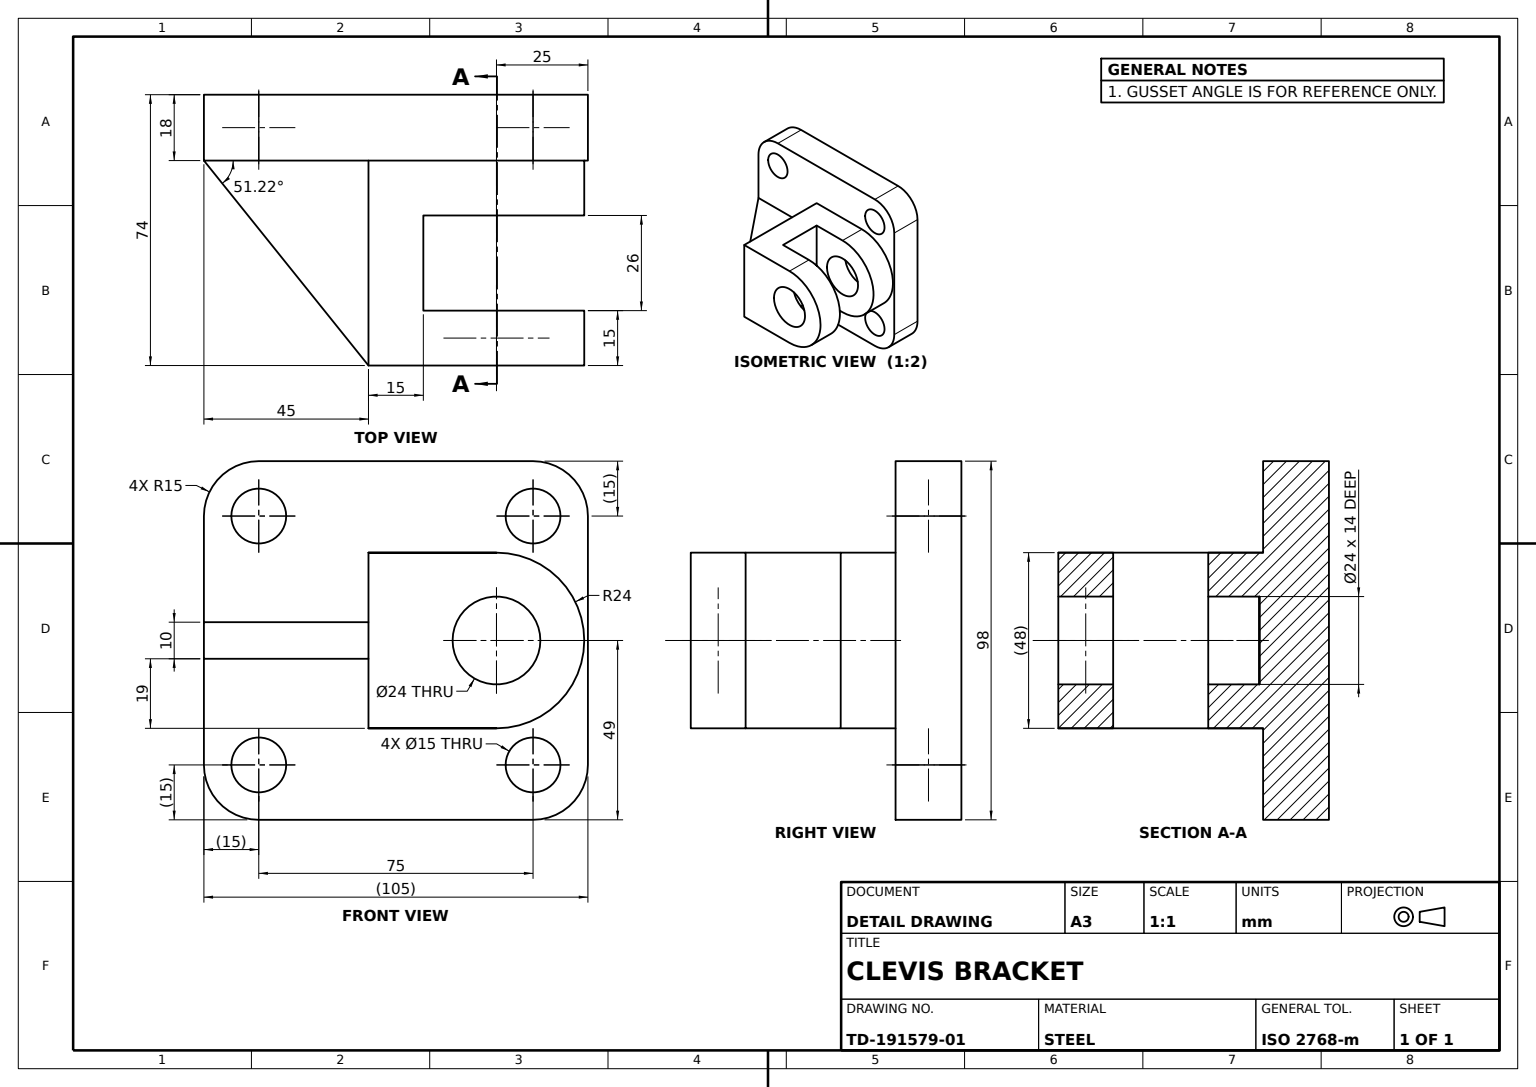
SolidWorks part; units mm, degrees
material "Plain Carbon Steel"
ref_plane "Front Plane" through (0, 0, 0) normal (0, 0, 1) x (1, 0, 0)
ref_plane "Top Plane" through (0, 0, 0) normal (0, 1, 0) x (1, 0, 0)
ref_plane "Right Plane" through (0, 0, 0) normal (1, 0, 0) x (0, 0, -1)
sketch "Base Plate Sketch" plane through (0, 0, 0) normal (0, 0, 1) x (1, 0, 0)
  line L0 (15, 0) -> (90, 0)
  line L1 (105, 15) -> (105, 83)
  line L2 (90, 98) -> (15, 98)
  line L3 (0, 83) -> (0, 15)
  arc A0 (15, 0) -> (0, 15) centre (15, 15) cw
  arc A1 (105, 15) -> (90, 0) centre (90, 15) cw
  arc A2 (105, 83) -> (90, 98) centre (90, 83) ccw
  arc A3 (0, 83) -> (15, 98) centre (15, 83) cw
  point P7 (0, 0)
  dimension "D1" = 15
  dimension "D2" = 105
  dimension "D3" = 98
extrude "Base Plate" add sketch "Base Plate Sketch" along normal blind 18
sketch "Mounting Holes Sketch" plane through (0, 0, 18) normal (0, 0, 1) x (1, 0, 0)
  circle A0 centre (15, 83) radius 7.5
  circle A1 centre (90, 83) radius 7.5
  circle A2 centre (90, 15) radius 7.5
  circle A3 centre (15, 15) radius 7.5
  dimension "D1" = 15
  dimension "D2" = 15
  dimension "D3" = 15
  dimension "D4" = 15
  dimension "D5" = 15
extrude "Mounting Holes 4xØ15" cut sketch "Mounting Holes Sketch" against normal blind 18
sketch "Clevis Base Boss Sketch" plane through (0, 0, 18) normal (0, 0, 1) x (1, 0, 0)
  line L0 (15, 0) -> (90, 0) construction
  line L3 (80, 73) -> (45, 73)
  line L4 (45, 73) -> (45, 25)
  line L5 (45, 25) -> (80, 25)
  arc A0 (80, 25) -> (80, 73) centre (80, 49) ccw
  dimension "D1" = 24
  dimension "D2" = 10
  dimension "D3" = 45
  dimension "D4" = 49
extrude "Clevis Base Boss" add sketch "Clevis Base Boss Sketch" along normal blind 15
sketch "Clevis Body Sketch" plane through (0, 25, 0) normal (0, -1, 0) x (1, 0, 0)
  line L0 (45, 33) -> (45, 74)
  line L1 (45, 74) -> (55, 74)
  line L2 (55, 74) -> (55, 33)
  line L3 (45, 33) -> (80, 33) construction
  line L4 (55, 33) -> (45, 33)
  line L5 (80, 33) -> (80, 18) construction
  line L6 (45, 18) -> (80, 18) construction
  dimension "D1" = 25
  dimension "D2" = 56
extrude "Clevis Body" add sketch "Clevis Body Sketch" against normal blind 48
sketch "Eye Spacer Sketch" plane through (55, 0, 0) normal (1, 0, 0) x (0, 0, -1)
  line L0 (-74, 73) -> (-74, 25)
  line L1 (-74, 25) -> (-33, 25)
  line L2 (-33, 25) -> (-33, 73)
  line L3 (-33, 73) -> (-74, 73)
extrude "Eye Spacer" add sketch "Eye Spacer Sketch" along normal blind 5
sketch "Eye Lug Sketch" plane through (0, 0, 74) normal (0, 0, 1) x (1, 0, 0)
  line L0 (60, 73) -> (80, 73)
  line L1 (80, 73) -> (80, 25)
  line L2 (80, 25) -> (60, 25)
  line L3 (60, 25) -> (60, 73)
extrude "Eye Lug" add sketch "Eye Lug Sketch" against normal blind 15
sketch "Eye Lug Round End Sketch" plane through (0, 0, 74) normal (0, 0, 1) x (1, 0, 0)
  line L0 (80, 25) -> (80, 73) construction
  line L1 (80, 73) -> (80, 25)
  arc A0 (80, 25) -> (80, 73) centre (80, 49) ccw
extrude "Eye Lug Round End" add sketch "Eye Lug Round End Sketch" against normal blind 15
sketch "Eye Bore Sketch" plane through (0, 0, 74) normal (0, 0, 1) x (1, 0, 0)
  circle A0 centre (80, 49) radius 12
  dimension "D1" = 24
  dimension "D2" = 24
extrude "Eye Bore Ø24" cut sketch "Eye Bore Sketch" against normal blind 55
sketch "Gusset Sketch" plane through (0, 25, 0) normal (0, -1, 0) x (1, 0, 0)
  line L0 (45, 74) -> (45, 18)
  line L1 (45, 18) -> (0, 18)
  line L2 (15, 18) -> (0, 18) construction
  line L3 (0, 18) -> (0, 0) construction
  line L4 (0, 18) -> (45, 74)
extrude "Gusset" add sketch "Gusset Sketch" against normal blind 48
sketch "Gusset Trim A Sketch" plane through (0, 25, 0) normal (0, -1, 0) x (1, 0, 0)
  line L0 (45, 74) -> (45, 18)
  line L1 (15, 18) -> (90, 18) construction
  line L2 (45, 18) -> (0, 18)
  line L3 (0, 18) -> (45, 74)
extrude "Gusset Trim A" cut sketch "Gusset Trim A Sketch" against normal blind 19
sketch "Gusset Trim B Sketch" plane through (0, 73, 0) normal (0, 1, 0) x (1, 0, 0)
  line L0 (45, -74) -> (45, -18)
  line L1 (90, -18) -> (15, -18) construction
  line L2 (45, -18) -> (0, -18)
  line L3 (0, -18) -> (45, -74)
extrude "Gusset Trim B" cut sketch "Gusset Trim B Sketch" against normal blind 19
